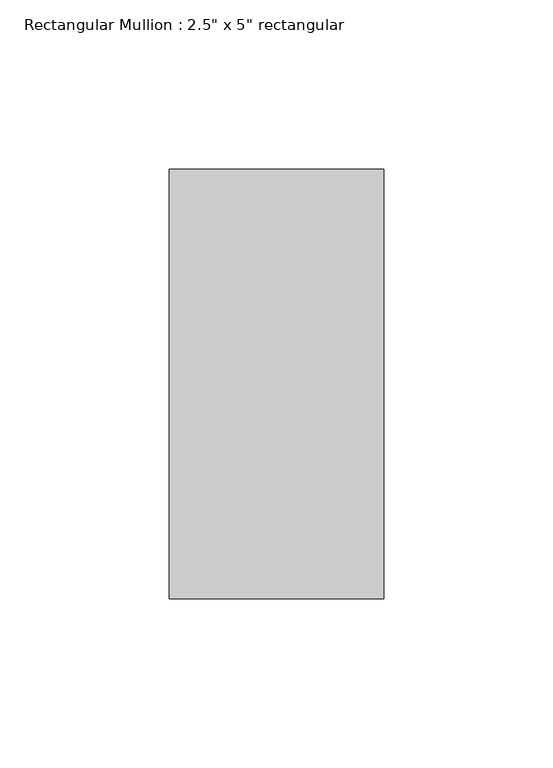
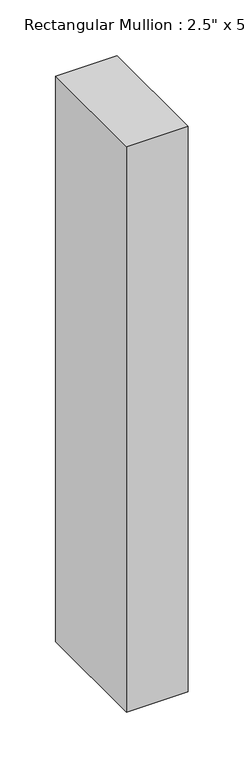
"""IFC4 building model written with IfcOpenShell, lengths in millimetres: member geometry."""

from ifc_helpers import new_model, si_unit, frame, origin, place, context, project, spatial, polyline, outline, extrude, source, transform, mapped, element, save


def member_2cd1b1d9(model_context):
    return source(origin(), model_context, "Body", "SweptSolid", [
        extrude(outline(polyline([(31.75, 63.5), (31.75, -63.5), (-31.75, -63.5), (-31.75, 63.5), (31.75, 63.5)])), frame((0.0, 0.0, -618.0666667), z_axis=(0.0, 0.0, 1.0), x_axis=(1.0, 0.0, 0.0)), (0.0, 0.0, 1.0), 618.0666667),
    ])


if __name__ == "__main__":
    model = new_model("IFC4")
    model_context = context("Model", 3, world=origin())
    ifc_project = project(units=[si_unit("LENGTHUNIT", "METRE", prefix="MILLI")], contexts=[model_context])
    site = spatial("IfcSite", under=ifc_project)
    building = spatial("IfcBuilding", under=site)
    placement = place(None, origin())
    member_shape = member_2cd1b1d9(model_context)
    element("IfcMember", 1, ObjectType="Rectangular Mullion : 2.5\" x 5\" rectangular", at=placement, inside=building, context=model_context, shape_type="MappedRepresentation", body=[
        mapped(member_shape, transform((0.0, 0.0, 0.0), x_axis=(1.0, 0.0, 0.0), y_axis=(0.0, 1.0, 0.0), z_axis=(0.0, 0.0, 1.0))),
    ])
    save(model, "model.ifc")

# Revit data of these elements
# Type "Rectangular Mullion : 2.5\" x 5\" rectangular"
#   built-in parameter 1007304 = 0.416667 (stored number, unit not read)
#   built-in parameter 1007301 = 0.104167 (stored number, unit not read)
#   built-in parameter 1007300 = 0.104167 (stored number, unit not read)
# Element 1 (IfcMember, "Rectangular Mullion : 2.5\" x 5\" rectangular")
#   Materials on its faces: "Door - Frame"
# Materials
#   "Door - Frame": colour RGB 118 70 51, transparency 0, Cost = 0
